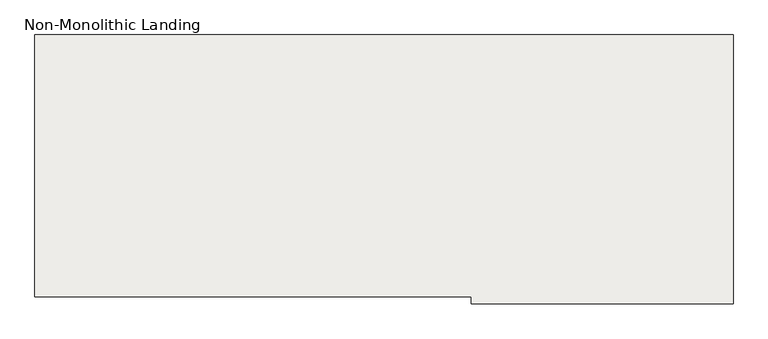
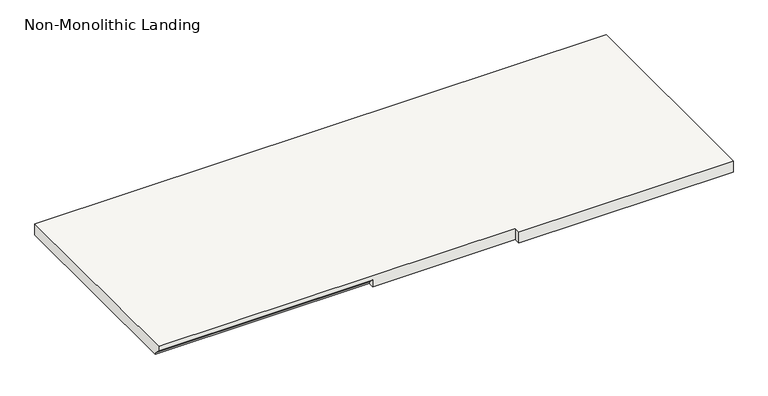
"""IFC4 building model written with IfcOpenShell, lengths in millimetres: slab geometry, Non-Monolithic Landing."""

from ifc_helpers import new_model, si_unit, origin, place, context, project, spatial, faceted_brep, source, transform, mapped, element, save


def non_monolithic_landing_47fb7adf(model_context):
    return source(origin(), model_context, "Body", "Brep", [
        faceted_brep([(-7672.6994093, 5734.2237487, 1664.2772727), (-7672.6994093, 5759.6237487, 1638.8772727), (-6758.2994093, 5759.6237487, 1638.8772727), (-6758.2994093, 5734.2237487, 1664.2772727), (-6148.6994093, 5734.2237487, 1683.3272727), (-6148.6994093, 5708.8237487, 1683.3272727), (-5234.2994093, 5708.8237487, 1683.3272727), (-5234.2994093, 5734.2237487, 1683.3272727), (-5234.2994093, 6648.6237487, 1683.3272727), (-7672.6994093, 6648.6237487, 1683.3272727), (-7672.6994093, 5734.2237487, 1683.3272727), (-6758.2994093, 5759.6237487, 1632.5272727), (-7672.6994093, 5759.6237487, 1632.5272727), (-7672.6994093, 6648.6237487, 1632.5272727), (-5234.2994093, 6648.6237487, 1632.5272727), (-5234.2994093, 5734.2237487, 1632.5272727), (-5234.2994093, 5708.8237487, 1632.5272727), (-6148.6994093, 5708.8237487, 1632.5272727), (-6148.6994093, 5734.2237487, 1632.5272727), (-6758.2994093, 5734.2237487, 1632.5272727)], [[[0, 1, 2, 3]], [[4, 5, 6, 7, 8, 9, 10]], [[11, 12, 13, 14, 15, 16, 17, 18, 19]], [[12, 11, 2, 1]], [[11, 19, 3, 2]], [[4, 10, 0, 3, 19, 18]], [[5, 4, 18, 17]], [[6, 5, 17, 16]], [[7, 6, 16, 15]], [[8, 7, 15, 14]], [[9, 8, 14, 13]], [[10, 9, 13, 12, 1, 0]]]),
    ])


if __name__ == "__main__":
    model = new_model("IFC4")
    model_context = context("Model", 3, world=origin())
    ifc_project = project(units=[si_unit("LENGTHUNIT", "METRE", prefix="MILLI")], contexts=[model_context])
    site = spatial("IfcSite", under=ifc_project)
    building = spatial("IfcBuilding", under=site)
    placement = place(None, origin())
    non_monolithic_landing_shape = non_monolithic_landing_47fb7adf(model_context)
    element("IfcSlab", 1, ObjectType="Non-Monolithic Landing", at=placement, inside=building, context=model_context, shape_type="MappedRepresentation", body=[
        mapped(non_monolithic_landing_shape, transform((0.0, 0.0, 0.0), x_axis=(1.0, 0.0, 0.0), y_axis=(0.0, 1.0, 0.0), z_axis=(0.0, 0.0, 1.0))),
    ])
    save(model, "model.ifc")
